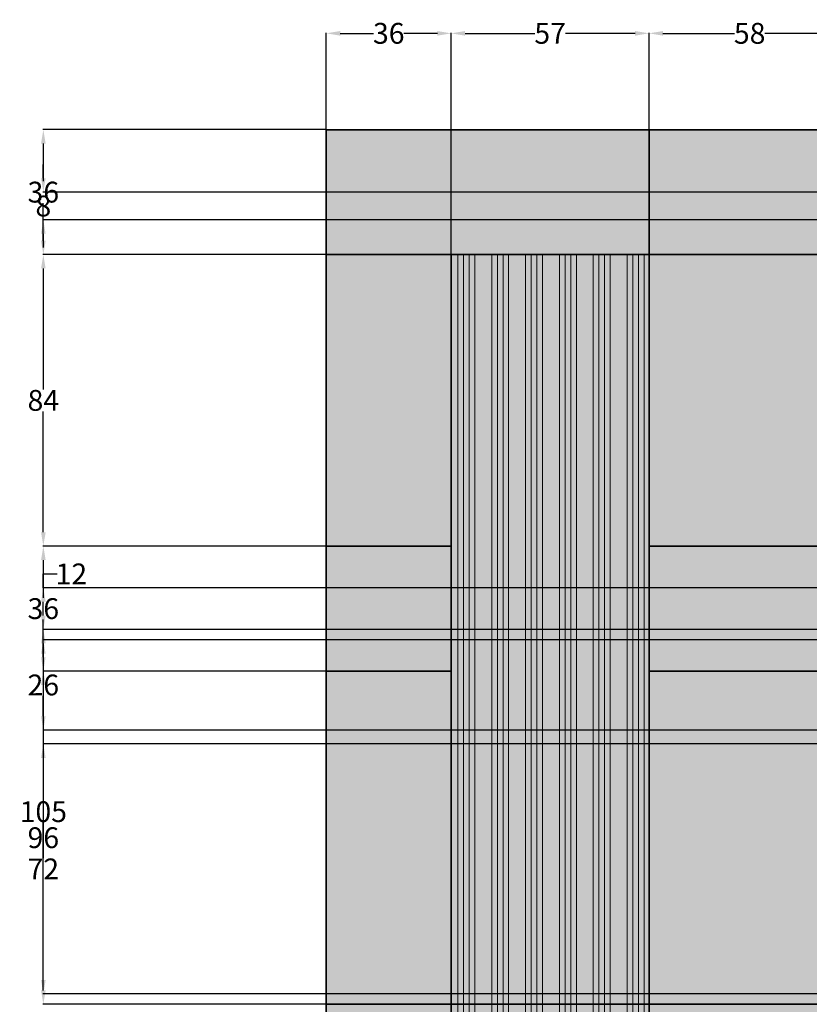
# Model space of a CAD drawing. Units: inches. Extents: x 221 to 874, y 171 to 738.
# Tile 4 of 11: x 225 to 452, y 455 to 738. Entities that reach past the tile are written whole.
import ezdxf

# ---------------------------------------------------------------- set-up
doc = ezdxf.new("R2010")
doc.units = ezdxf.units.IN
doc.header["$MEASUREMENT"] = 0
for name, color, linetype, lineweight in [('A-ANNO-DIMS', 2, 'Continuous', 18), ('A-ELEV', 7, 'Continuous', 35), ('A-ELEV-PATT', 8, 'Continuous', 13)]:
    doc.layers.add(name, color=color, linetype=linetype, lineweight=lineweight)
doc.styles.get("Standard").update_dxf_attribs({"font": 'arial.ttf'})
doc.dimstyles.get("Standard").update_dxf_attribs({"dimtxt": 6, "dimasz": 4, "dimexe": 0.18, "dimexo": 0.0625, "dimgap": 0.09, "dimtad": 0, "dimtih": 1, "dimtoh": 1, "dimdec": 0, "dimzin": 0, "dimdsep": 46, "dimlunit": 3, "dimtxsty": 'Standard', "dimcen": 0.09, "dimadec": 0, "dimazin": 0, "dimtfac": 1, "dimtdec": 0, "dimtofl": 0, "dimtmove": 0, "dimatfit": 3, "dimfxl": 1, "dimtolj": 1, "dimtzin": 0, "dimarcsym": 0})

# ---------------------------------------------------------------- blocks, each defined once
blk = doc.blocks.new('*D22')
at = {"layer": 'A-ANNO-DIMS', "color": 0, "lineweight": -2, "transparency": 16777216}
for p, q in [((313.08, 670.78), (313.08, 734.65)), ((317.08, 734.47), (326.7, 734.47)), ((345.08, 734.47), (335.46, 734.47)), ((349.08, 670.78), (349.08, 734.65))]:
    blk.add_line(p, q, dxfattribs=at)
at = {"layer": 'A-ANNO-DIMS', "color": 0, "transparency": 16777216}
for points in [[(317.08, 735.13), (317.08, 733.8), (313.08, 734.47)], [(345.08, 735.13), (345.08, 733.8), (349.08, 734.47)]]:
    blk.add_solid(points, dxfattribs=at)
at = {"layer": 'Defpoints', "color": 0, "transparency": 16777216}
for p in [(349.08, 734.47), (313.08, 670.72), (349.08, 670.72)]:
    blk.add_point(p, dxfattribs=at)
at = {"layer": 'A-ANNO-DIMS', "color": 0, "transparency": 16777216, "insert": (331.08, 734.47), "char_height": 6, "attachment_point": 5}
blk.add_mtext('\\A1;36', dxfattribs=at)
blk = doc.blocks.new('*D23')
at = {"layer": 'A-ANNO-DIMS', "color": 0, "lineweight": -2, "transparency": 16777216}
for p, q in [((349.08, 670.78), (349.08, 734.65)), ((353.08, 734.47), (373.19, 734.47)), ((402.08, 734.47), (381.97, 734.47)), ((406.08, 670.78), (406.08, 734.65))]:
    blk.add_line(p, q, dxfattribs=at)
at = {"layer": 'A-ANNO-DIMS', "color": 0, "transparency": 16777216}
for points in [[(353.08, 735.13), (353.08, 733.8), (349.08, 734.47)], [(402.08, 735.13), (402.08, 733.8), (406.08, 734.47)]]:
    blk.add_solid(points, dxfattribs=at)
at = {"layer": 'Defpoints', "color": 0, "transparency": 16777216}
for p in [(406.08, 734.47), (349.08, 670.72), (406.08, 670.72)]:
    blk.add_point(p, dxfattribs=at)
at = {"layer": 'A-ANNO-DIMS', "color": 0, "transparency": 16777216, "insert": (377.58, 734.47), "char_height": 6, "attachment_point": 5}
blk.add_mtext('\\A1;57', dxfattribs=at)
blk = doc.blocks.new('*D24')
at = {"layer": 'A-ANNO-DIMS', "color": 0, "lineweight": -2, "transparency": 16777216}
for p, q in [((406.08, 706.78), (406.08, 734.65)), ((410.08, 734.47), (430.69, 734.47)), ((460.08, 734.47), (439.47, 734.47)), ((464.08, 706.78), (464.08, 734.65))]:
    blk.add_line(p, q, dxfattribs=at)
at = {"layer": 'A-ANNO-DIMS', "color": 0, "transparency": 16777216}
for points in [[(410.08, 735.13), (410.08, 733.8), (406.08, 734.47)], [(460.08, 735.13), (460.08, 733.8), (464.08, 734.47)]]:
    blk.add_solid(points, dxfattribs=at)
at = {"layer": 'Defpoints', "color": 0, "transparency": 16777216}
for p in [(464.08, 734.47), (406.08, 706.72), (464.08, 706.72)]:
    blk.add_point(p, dxfattribs=at)
at = {"layer": 'A-ANNO-DIMS', "color": 0, "transparency": 16777216, "insert": (435.08, 734.47), "char_height": 6, "attachment_point": 5}
blk.add_mtext('\\A1;58', dxfattribs=at)
blk = doc.blocks.new('*D36')
at = {"layer": 'A-ANNO-DIMS', "color": 0, "lineweight": -2, "transparency": 16777216}
for p, q in [((313.02, 550.72), (231.36, 550.72)), ((231.54, 546.72), (231.54, 505.87)), ((231.54, 458.72), (231.54, 499.56)), ((313.02, 454.72), (231.36, 454.72))]:
    blk.add_line(p, q, dxfattribs=at)
at = {"layer": 'A-ANNO-DIMS', "color": 0, "transparency": 16777216}
for points in [[(230.88, 546.72), (232.21, 546.72), (231.54, 550.72)], [(230.88, 458.72), (232.21, 458.72), (231.54, 454.72)]]:
    blk.add_solid(points, dxfattribs=at)
at = {"layer": 'Defpoints', "color": 0, "transparency": 16777216}
for p in [(231.54, 550.72), (313.08, 550.72), (313.08, 454.72)]:
    blk.add_point(p, dxfattribs=at)
at = {"layer": 'A-ANNO-DIMS', "color": 0, "transparency": 16777216, "insert": (231.54, 502.72), "char_height": 6, "attachment_point": 5}
blk.add_mtext('\\A1;96', dxfattribs=at)
blk = doc.blocks.new('*D37')
at = {"layer": 'A-ANNO-DIMS', "color": 0, "lineweight": -2, "transparency": 16777216}
for p, q in [((313.02, 586.72), (231.36, 586.72)), ((231.54, 582.72), (231.54, 571.87)), ((231.54, 554.72), (231.54, 565.56)), ((313.02, 550.72), (231.36, 550.72))]:
    blk.add_line(p, q, dxfattribs=at)
at = {"layer": 'A-ANNO-DIMS', "color": 0, "transparency": 16777216}
for points in [[(230.88, 582.72), (232.21, 582.72), (231.54, 586.72)], [(230.88, 554.72), (232.21, 554.72), (231.54, 550.72)]]:
    blk.add_solid(points, dxfattribs=at)
at = {"layer": 'Defpoints', "color": 0, "transparency": 16777216}
for p in [(231.54, 586.72), (313.08, 586.72), (313.08, 550.72)]:
    blk.add_point(p, dxfattribs=at)
at = {"layer": 'A-ANNO-DIMS', "color": 0, "transparency": 16777216, "insert": (231.54, 568.72), "char_height": 6, "attachment_point": 5}
blk.add_mtext('\\A1;36', dxfattribs=at)
blk = doc.blocks.new('*D38')
at = {"layer": 'A-ANNO-DIMS', "color": 0, "lineweight": -2, "transparency": 16777216}
for p, q in [((313.02, 670.72), (231.36, 670.72)), ((231.54, 666.72), (231.54, 631.87)), ((231.54, 590.72), (231.54, 625.56)), ((313.02, 586.72), (231.36, 586.72))]:
    blk.add_line(p, q, dxfattribs=at)
at = {"layer": 'A-ANNO-DIMS', "color": 0, "transparency": 16777216}
for points in [[(230.88, 666.72), (232.21, 666.72), (231.54, 670.72)], [(230.88, 590.72), (232.21, 590.72), (231.54, 586.72)]]:
    blk.add_solid(points, dxfattribs=at)
at = {"layer": 'Defpoints', "color": 0, "transparency": 16777216}
for p in [(231.54, 670.72), (313.08, 670.72), (313.08, 586.72)]:
    blk.add_point(p, dxfattribs=at)
at = {"layer": 'A-ANNO-DIMS', "color": 0, "transparency": 16777216, "insert": (231.54, 628.72), "char_height": 6, "attachment_point": 5}
blk.add_mtext('\\A1;84', dxfattribs=at)
blk = doc.blocks.new('*D39')
at = {"layer": 'A-ANNO-DIMS', "color": 0, "lineweight": -2, "transparency": 16777216}
for p, q in [((313.02, 706.72), (231.36, 706.72)), ((231.54, 702.72), (231.54, 691.87)), ((231.54, 674.72), (231.54, 685.56)), ((313.02, 670.72), (231.36, 670.72))]:
    blk.add_line(p, q, dxfattribs=at)
at = {"layer": 'A-ANNO-DIMS', "color": 0, "transparency": 16777216}
for points in [[(230.88, 702.72), (232.21, 702.72), (231.54, 706.72)], [(230.88, 674.72), (232.21, 674.72), (231.54, 670.72)]]:
    blk.add_solid(points, dxfattribs=at)
at = {"layer": 'Defpoints', "color": 0, "transparency": 16777216}
for p in [(231.54, 706.72), (313.08, 706.72), (313.08, 670.72)]:
    blk.add_point(p, dxfattribs=at)
at = {"layer": 'A-ANNO-DIMS', "color": 0, "transparency": 16777216, "insert": (231.54, 688.72), "char_height": 6, "attachment_point": 5}
blk.add_mtext('\\A1;36', dxfattribs=at)
blk = doc.blocks.new('*D40')
at = {"layer": 'A-ANNO-DIMS', "color": 0, "lineweight": -2, "transparency": 16777216}
for p, q in [((231.54, 692.72), (231.54, 696.72)), ((464.02, 688.72), (231.36, 688.72)), ((464.02, 680.72), (231.36, 680.72)), ((231.54, 676.72), (231.54, 672.72))]:
    blk.add_line(p, q, dxfattribs=at)
at = {"layer": 'A-ANNO-DIMS', "color": 0, "transparency": 16777216}
for points in [[(230.88, 692.72), (232.21, 692.72), (231.54, 688.72)], [(230.88, 676.72), (232.21, 676.72), (231.54, 680.72)]]:
    blk.add_solid(points, dxfattribs=at)
at = {"layer": 'Defpoints', "color": 0, "transparency": 16777216}
for p in [(231.54, 688.72), (464.08, 688.72), (464.08, 680.72)]:
    blk.add_point(p, dxfattribs=at)
at = {"layer": 'A-ANNO-DIMS', "color": 0, "transparency": 16777216, "insert": (231.54, 684.72), "char_height": 6, "attachment_point": 5}
blk.add_mtext('\\A1;8', dxfattribs=at)
blk = doc.blocks.new('*D51')
at = {"layer": 'A-ANNO-DIMS', "color": 0, "lineweight": -2, "transparency": 16777216}
for p, q in [((546.29, 562.72), (231.36, 562.72)), ((231.54, 558.72), (231.54, 513.37)), ((231.54, 461.72), (231.54, 507.06)), ((546.29, 457.72), (231.36, 457.72))]:
    blk.add_line(p, q, dxfattribs=at)
at = {"layer": 'A-ANNO-DIMS', "color": 0, "transparency": 16777216}
for points in [[(230.88, 558.72), (232.21, 558.72), (231.54, 562.72)], [(230.88, 461.72), (232.21, 461.72), (231.54, 457.72)]]:
    blk.add_solid(points, dxfattribs=at)
at = {"layer": 'Defpoints', "color": 0, "transparency": 16777216}
for p in [(231.54, 562.72), (546.35, 562.72), (546.35, 457.72)]:
    blk.add_point(p, dxfattribs=at)
at = {"layer": 'A-ANNO-DIMS', "color": 0, "transparency": 16777216, "insert": (231.54, 510.22), "char_height": 6, "attachment_point": 5}
blk.add_mtext('\\A1;105', dxfattribs=at)
blk = doc.blocks.new('*D52')
at = {"layer": 'A-ANNO-DIMS', "color": 0, "lineweight": -2, "transparency": 16777216}
for p, q in [((231.54, 574.72), (231.54, 578.72)), ((231.54, 578.72), (235.54, 578.72)), ((546.29, 574.72), (231.36, 574.72)), ((231.54, 566.72), (231.54, 570.72)), ((546.29, 562.72), (231.36, 562.72))]:
    blk.add_line(p, q, dxfattribs=at)
at = {"layer": 'A-ANNO-DIMS', "color": 0, "transparency": 16777216}
for points in [[(230.88, 570.72), (232.21, 570.72), (231.54, 574.72)], [(230.88, 566.72), (232.21, 566.72), (231.54, 562.72)]]:
    blk.add_solid(points, dxfattribs=at)
at = {"layer": 'Defpoints', "color": 0, "transparency": 16777216}
for p in [(231.54, 574.72), (546.35, 574.72), (546.35, 562.72)]:
    blk.add_point(p, dxfattribs=at)
at = {"layer": 'A-ANNO-DIMS', "color": 0, "transparency": 16777216, "insert": (239.62, 578.72), "char_height": 6, "attachment_point": 5}
blk.add_mtext('\\A1;12', dxfattribs=at)
blk = doc.blocks.new('*D55')
at = {"layer": 'A-ANNO-DIMS', "color": 0, "lineweight": -2, "transparency": 16777216}
for p, q in [((754.02, 559.72), (231.36, 559.72)), ((231.54, 555.72), (231.54, 549.87)), ((231.54, 537.72), (231.54, 543.56)), ((754.02, 533.72), (231.36, 533.72))]:
    blk.add_line(p, q, dxfattribs=at)
at = {"layer": 'A-ANNO-DIMS', "color": 0, "transparency": 16777216}
for points in [[(230.88, 555.72), (232.21, 555.72), (231.54, 559.72)], [(230.88, 537.72), (232.21, 537.72), (231.54, 533.72)]]:
    blk.add_solid(points, dxfattribs=at)
at = {"layer": 'Defpoints', "color": 0, "transparency": 16777216}
for p in [(231.54, 559.72), (754.08, 559.72), (754.08, 533.72)]:
    blk.add_point(p, dxfattribs=at)
at = {"layer": 'A-ANNO-DIMS', "color": 0, "transparency": 16777216, "insert": (231.54, 546.72), "char_height": 6, "attachment_point": 5}
blk.add_mtext('\\A1;26', dxfattribs=at)
blk = doc.blocks.new('*D56')
at = {"layer": 'A-ANNO-DIMS', "color": 0, "lineweight": -2, "transparency": 16777216}
for p, q in [((754.02, 529.72), (231.36, 529.72)), ((231.54, 525.72), (231.54, 496.82)), ((231.54, 461.72), (231.54, 490.61)), ((754.02, 457.72), (231.36, 457.72))]:
    blk.add_line(p, q, dxfattribs=at)
at = {"layer": 'A-ANNO-DIMS', "color": 0, "transparency": 16777216}
for points in [[(230.88, 525.72), (232.21, 525.72), (231.54, 529.72)], [(230.88, 461.72), (232.21, 461.72), (231.54, 457.72)]]:
    blk.add_solid(points, dxfattribs=at)
at = {"layer": 'Defpoints', "color": 0, "transparency": 16777216}
for p in [(231.54, 529.72), (754.08, 529.72), (754.08, 457.72)]:
    blk.add_point(p, dxfattribs=at)
at = {"layer": 'A-ANNO-DIMS', "color": 0, "transparency": 16777216, "insert": (231.54, 493.72), "char_height": 6, "attachment_point": 5}
blk.add_mtext('\\A1;72', dxfattribs=at)

msp = doc.modelspace()

# ---------------------------------------------------------------- hatches: boundary and pattern name
at = {"layer": 'A-ELEV-PATT'}
h = msp.add_hatch(color=256, dxfattribs=at)
h.dxf.hatch_style = 1
h.paths.add_polyline_path([(349.0786, 286.1996), (313.0786, 286.1996), (313.0786, 232.7164), (349.0786, 232.7164)])
h.paths.add_polyline_path([(464.0786, 286.1996), (406.0786, 286.1996), (406.0786, 232.7164), (464.0786, 232.7164)])
h.paths.add_polyline_path([(541.0786, 286.1996), (493.0786, 286.1996), (493.0786, 232.7164), (541.0786, 232.7164)])
h.paths.add_polyline_path([(541.0786, 370.7164), (493.0786, 370.7164), (493.0786, 286.1996), (541.0786, 286.1996)])
h.paths.add_polyline_path([(464.0786, 370.7164), (406.0786, 370.7164), (406.0786, 286.1996), (464.0786, 286.1996)])
h.paths.add_polyline_path([(349.0786, 370.7164), (313.0786, 370.7164), (313.0786, 286.1996), (349.0786, 286.1996)])
h.paths.add_polyline_path([(349.0786, 454.7164), (313.0786, 454.7164), (313.0786, 370.7164), (349.0786, 370.7164)])
h.paths.add_polyline_path([(464.0786, 454.7164), (406.0786, 454.7164), (406.0786, 370.7164), (464.0786, 370.7164)])
h.paths.add_polyline_path([(541.0786, 418.7164), (541.0786, 454.7164), (493.0786, 454.7164), (493.0786, 370.7164), (541.0786, 370.7164)])
h.paths.add_polyline_path([(541.0786, 550.7164), (493.0786, 550.7164), (493.0786, 454.7164), (541.0786, 454.7164)])
h.paths.add_polyline_path([(464.0786, 550.7164), (406.0786, 550.7164), (406.0786, 454.7164), (464.0786, 454.7164)])
h.paths.add_polyline_path([(349.0786, 550.7164), (313.0786, 550.7164), (313.0786, 454.7164), (349.0786, 454.7164)])
h.paths.add_polyline_path([(349.0786, 586.7164), (313.0786, 586.7164), (313.0786, 550.7164), (349.0786, 550.7164)])
h.paths.add_polyline_path([(464.0786, 586.7164), (406.0786, 586.7164), (406.0786, 550.7164), (464.0786, 550.7164)])
h.paths.add_polyline_path([(541.0786, 574.7164), (541.0786, 586.7164), (493.0786, 586.7164), (493.0786, 550.7164), (541.0786, 550.7164)])
h.paths.add_polyline_path([(541.0786, 670.7164), (493.0786, 670.7164), (493.0786, 586.7164), (541.0786, 586.7164)])
h.paths.add_polyline_path([(464.0786, 670.7164), (406.0786, 670.7164), (406.0786, 586.7164), (464.0786, 586.7164)])
h.paths.add_polyline_path([(349.0786, 670.7164), (313.0786, 670.7164), (313.0786, 586.7164), (349.0786, 586.7164)])
h.paths.add_polyline_path([(406.0786, 706.7164), (313.0786, 706.7164), (313.0786, 670.7164), (349.0786, 670.7164), (406.0786, 670.7164)])
h.paths.add_polyline_path([(464.0786, 706.7164), (406.0786, 706.7164), (406.0786, 670.7164), (464.0786, 670.7164)])
h.paths.add_polyline_path([(541.0786, 706.7164), (493.0786, 706.7164), (493.0786, 688.7164), (493.0786, 670.7164), (541.0786, 670.7164)])
h.paths.add_polyline_path([(660.0786, 610.7164), (541.0786, 610.7164), (541.0786, 586.7164), (541.0786, 574.7164), (660.0786, 574.7164)])
h.paths.add_polyline_path([(781.0786, 610.7164), (660.0786, 610.7164), (660.0786, 574.7164), (769.0786, 574.7164), (781.0786, 574.7164)])
h.paths.add_polyline_path([(781.0786, 574.7164), (769.0786, 574.7164), (769.0786, 476.1199), (781.0786, 476.1199)])
h.paths.add_polyline_path([(781.0786, 476.1199), (769.0786, 476.1199), (769.0786, 457.7164), (781.0786, 457.7164)])
h.paths.add_polyline_path([(781.0786, 377.1023), (705.9097, 377.1023), (705.9097, 286.1996), (781.0786, 286.1996)])
h.paths.add_polyline_path([(741.9618, 338.8486), (756.9618, 338.8486), (756.9618, 329.8486), (741.9618, 329.8486)], flags=16)
h.paths.add_polyline_path([(648.9097, 377.1023), (598.0786, 377.1023), (598.0786, 286.1996), (648.9097, 286.1996)])
h.paths.add_polyline_path([(781.0786, 286.1996), (705.9097, 286.1996), (705.9097, 280.7164), (648.9097, 280.7164), (648.9097, 286.1996), (598.0786, 286.1996), (598.0786, 280.7164), (550.0786, 280.7164), (550.0786, 286.1996), (541.0786, 286.1996), (541.0786, 274.7164), (781.0786, 274.7164)])
h.paths.add_polyline_path([(660.0786, 562.7164), (546.3477, 562.7164), (546.3477, 457.7164), (660.0786, 457.7164)])
h = msp.add_hatch(color=256, dxfattribs=at)
h.paths.add_polyline_path([(406.0786, 670.7164), (349.0786, 670.7164), (349.0786, 454.7164), (406.0786, 454.7164)])
h.paths.add_polyline_path([(406.0786, 454.7164), (349.0786, 454.7164), (349.0786, 232.7164), (406.0786, 232.7164)])
h = msp.add_hatch(dxfattribs=at)
h.set_pattern_fill('ANSI34', color=256, scale=13, angle=45, style=0)
h.paths.add_polyline_path([(406.0786, 670.7164), (349.0786, 670.7164), (349.0786, 454.7164), (406.0786, 454.7164)])
h.paths.add_polyline_path([(406.0786, 454.7164), (349.0786, 454.7164), (349.0786, 232.7164), (406.0786, 232.7164)])

# ---------------------------------------------------------------- linework, layer by layer
at = {"layer": 'A-ELEV'}
for p, q in [((313.0786, 706.7164), (464.0786, 706.7164)), ((313.0786, 232.7164), (313.0786, 706.7164)), ((406.0786, 670.7164), (406.0786, 706.7164)), ((313.0786, 670.7164), (464.0786, 670.7164)), ((349.0786, 232.7164), (349.0786, 670.7164)), ((406.0786, 232.7164), (406.0786, 670.7164)), ((313.0786, 586.7164), (349.0786, 586.7164)), ((406.0786, 586.7164), (464.0786, 586.7164)), ((313.0786, 550.7164), (349.0786, 550.7164)), ((406.0786, 550.7164), (464.0786, 550.7164)), ((313.0786, 454.7164), (464.0786, 454.7164))]:
    msp.add_line(p, q, dxfattribs=at)

# ---------------------------------------------------------------- dimensions: what is measured, and where the dimension line sits
at = {"layer": 'A-ANNO-DIMS'}
for base, p1, p2, picture, middle in [((349.0786, 734.4664), (313.0786, 670.7164), (349.0786, 670.7164), '*D22', (331.0786, 734.4664)), ((406.0786, 734.4664), (349.0786, 670.7164), (406.0786, 670.7164), '*D23', (377.5786, 734.4664)), ((464.0786, 734.4664), (406.0786, 706.7164), (464.0786, 706.7164), '*D24', (435.0786, 734.4664))]:
    dim = msp.add_linear_dim(base=base, p1=p1, p2=p2, dimstyle='Standard', override={"dimdec": 0, "dimlfac": 1, "dimrnd": 0, "dimzin": 0, "dimdsep": 46, "dimlunit": 2}, dxfattribs=at)
    dim.commit()
    dim.dimension.update_dxf_attribs({"geometry": picture, "text_midpoint": middle})
for base, p1, p2, picture, middle in [((231.5426, 706.7164), (313.0786, 670.7164), (313.0786, 706.7164), '*D39', (231.5426, 688.7164)), ((231.5426, 688.7164), (464.0786, 680.7164), (464.0786, 688.7164), '*D40', (231.5426, 684.7164)), ((231.5426, 670.7164), (313.0786, 586.7164), (313.0786, 670.7164), '*D38', (231.5426, 628.7164)), ((231.5426, 586.7164), (313.0786, 550.7164), (313.0786, 586.7164), '*D37', (231.5426, 568.7164)), ((231.5426, 574.7164), (546.3477, 562.7164), (546.3477, 574.7164), '*D52', (239.6169, 578.7164)), ((231.5426, 562.7164), (546.3477, 457.7164), (546.3477, 562.7164), '*D51', (231.5426, 510.2164)), ((231.5426, 559.7164), (754.0786, 533.7164), (754.0786, 559.7164), '*D55', (231.5426, 546.7164)), ((231.5426, 550.7164), (313.0786, 454.7164), (313.0786, 550.7164), '*D36', (231.5426, 502.7164)), ((231.5426, 529.7164), (754.0786, 457.7164), (754.0786, 529.7164), '*D56', (231.5426, 493.7164))]:
    dim = msp.add_linear_dim(base=base, p1=p1, p2=p2, angle=90, dimstyle='Standard', override={"dimdec": 0, "dimlfac": 1, "dimrnd": 0, "dimzin": 0, "dimdsep": 46, "dimlunit": 2}, dxfattribs=at)
    dim.commit()
    dim.dimension.update_dxf_attribs({"geometry": picture, "text_midpoint": middle})

doc.saveas('drawing.dxf')
